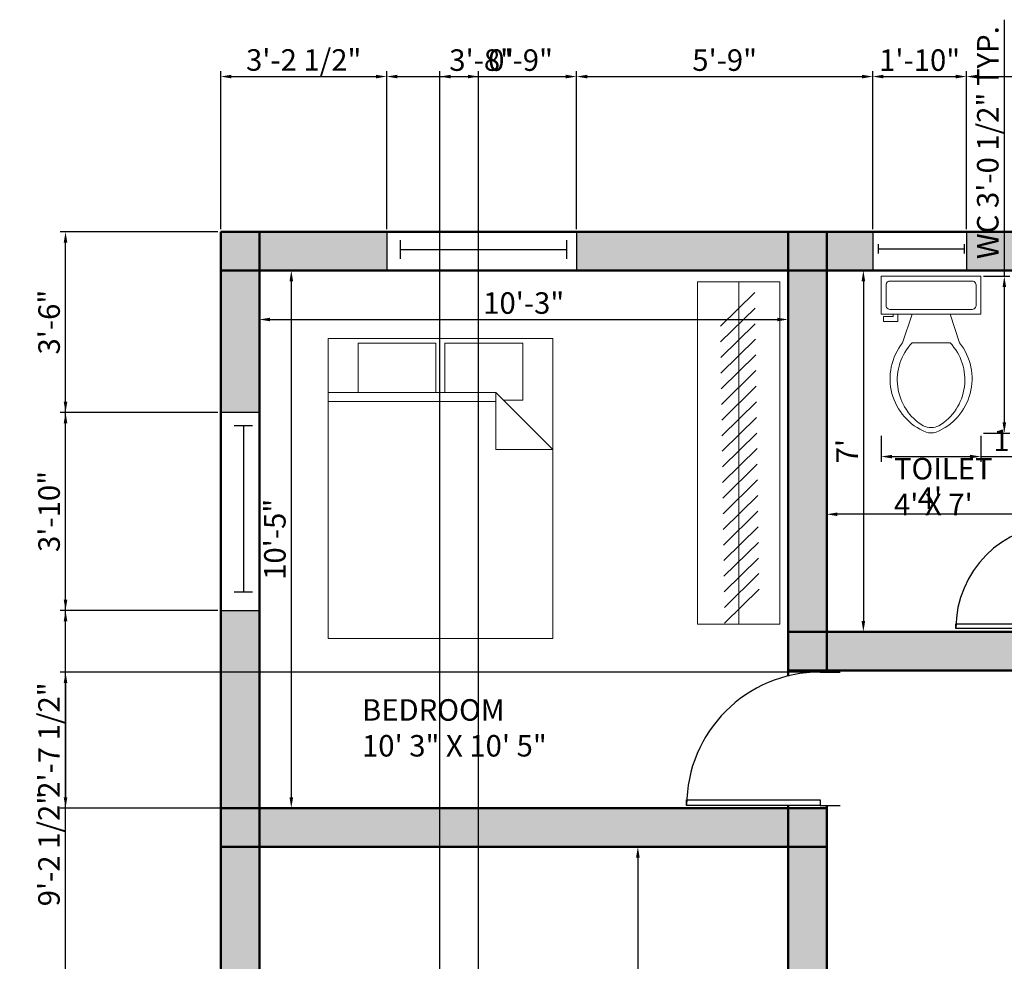
# Model space of a CAD drawing. Units: millimetres. Extents: x 2784 to 3697, y 603 to 1406.
# Tile 3 of 10: x 2784 to 3013, y 1187 to 1406. Entities that reach past the tile are written whole.
import ezdxf

# ---------------------------------------------------------------- set-up
doc = ezdxf.new("R2010")
doc.units = ezdxf.units.MM
for name, color, linetype, lineweight in [('A-ANNO-DIMS', 140, 'Continuous', 18), ('A-AREA-IDEN', 150, 'Continuous', 25), ('A-DOOR', 10, 'Continuous', 25), ('A-FLOR-FIXT', 8, 'Continuous', 18), ('A-FURN', 80, 'Continuous', 18), ('A-GLAZ', 30, 'Continuous', 25), ('A-WALL', 2, 'Continuous', 50), ('A-WALL-PATT', 8, 'Continuous', 13)]:
    doc.layers.add(name, color=color, linetype=linetype, lineweight=lineweight)
doc.styles.get("Standard").update_dxf_attribs({"font": 'arial.ttf'})
doc.dimstyles.new('ISO-25', dxfattribs={"dimtxt": 5, "dimasz": 2.5, "dimexe": 1.25, "dimexo": 0.625, "dimtad": 1, "dimdec": 0, "dimlunit": 3, "dimtxsty": 'Standard', "dimcen": 2.5, "dimadec": 0, "dimazin": 0, "dimtfac": 1, "dimtdec": 0, "dimtmove": 0, "dimatfit": 3, "dimfxl": 1, "dimarcsym": 0})

# ---------------------------------------------------------------- blocks, each defined once
blk = doc.blocks.new('*U2')
for p, q in [((0, 0), (0, -6)), ((40, 0), (40, -6))]:
    blk.add_line(p, q)
blk.add_lwpolyline([(0, 0), (0, 40), (1.75, 40), (1.75, 0)], close=True)
blk.add_arc((0, 0), 40, 0, 90)
blk = doc.blocks.new('*U4')
for p, q in [((0, 4), (0, 0)), ((36, 4), (36, 0)), ((0, 2), (36, 2))]:
    blk.add_line(p, q)
blk = doc.blocks.new('*U5')
for p, q in [((0, 4), (0, 0)), ((0, 2), (36, 2)), ((36, 4), (36, 0))]:
    blk.add_line(p, q)
blk = doc.blocks.new('Bed - Queen')
for p, q in [((0, -80.00003), (0, 0)), ((0, 0), (59.99999, 0)), ((59.99999, 0), (59.99999, -80.00003)), ((7.99999, -1.2), (28.79998, -1.2)), ((7.99999, -14.4), (7.99999, -1.2)), ((28.79998, -1.2), (28.79998, -14.4)), ((31.19999, -1.2), (51.99999, -1.2)), ((31.19999, -14.4), (31.19999, -1.2)), ((51.99999, -1.2), (51.99999, -16.4)), ((0, -14.4), (44.8, -14.4)), ((59.99999, -29.6), (44.8, -14.4)), ((44.8, -14.4), (44.8, -29.6)), ((44.8, -16.8), (0, -16.8)), ((51.99999, -16.4), (46.79936, -16.4)), ((44.8, -29.6), (59.99999, -29.6)), ((59.99999, -80.00003), (0, -80.00003))]:
    blk.add_line(p, q)
blk = doc.blocks.new('Toilet - top')
for p, q in [((9.5, -6), (9.5, -2)), ((-8, -8.5), (-8, -8)), ((-7, -8), (-7, -9.5)), ((-4, -8), (-6, -14)), ((4, -8), (6, -14)), ((-10, -8.5), (-8, -8.5)), ((-10, -9.5), (-10, -8.5)), ((-7, -9.5), (-10, -9.5)), ((4, -14), (-4, -14))]:
    blk.add_line(p, q)
blk.add_lwpolyline([(10.5, -8), (10.5, 0), (-10.5, 0), (-10.5, -8)], close=True)
for points in [[(-9.5, -2), (-9.5, -6)], [(8.5, -1), (-8.5, -1)], [(-8.5, -7), (8.5, -7)]]:
    blk.add_lwpolyline(points)
for centre, radius, start, end in [((-8.62, -1.88), 0.884, 81.8699, 188.1301), ((8.62, -1.88), 0.884, 351.8699, 98.1301), ((-8.62, -6.12), 0.884, 171.8699, 278.1301), ((8.62, -6.12), 0.884, 261.8699, 8.1301), ((3.52, -21.58), 12.17, 141.4691, 247.9714), ((4.2, -21.82), 11.33, 136.3677, 238.9468), ((-3.52, -21.58), 12.17, 292.0284, 38.5307), ((-4.2, -21.82), 11.33, 301.053, 43.6321), ((0, -27.88), 4, 245.7318, 294.2682), ((0, -29), 4, 254.8605, 285.1395)]:
    blk.add_arc(centre, radius, start, end)
blk = doc.blocks.new('*D15')
at = {"layer": 'A-ANNO-DIMS', "color": 0, "lineweight": -2, "transparency": 16777216}
for p, q in [((2847.96, 1347.23), (2848.58, 1347.23)), ((2847.33, 1344.73), (2847.33, 1224.73)), ((2847.96, 1222.23), (2848.58, 1222.23))]:
    blk.add_line(p, q, dxfattribs=at)
at = {"layer": 'A-ANNO-DIMS', "color": 0, "transparency": 16777216}
for points in [[(2846.92, 1344.73), (2847.75, 1344.73), (2847.33, 1347.23)], [(2846.92, 1224.73), (2847.75, 1224.73), (2847.33, 1222.23)]]:
    blk.add_solid(points, dxfattribs=at)
at = {"layer": 'Defpoints', "color": 0, "transparency": 16777216}
for p in [(2847.33, 1347.23), (2847.33, 1222.23), (2847.33, 1222.23)]:
    blk.add_point(p, dxfattribs=at)
at = {"layer": 'A-ANNO-DIMS', "color": 0, "transparency": 16777216, "insert": (2844.16, 1284.73), "char_height": 5, "attachment_point": 5, "rotation": 90}
blk.add_mtext('10\'-5"', dxfattribs=at)
blk = doc.blocks.new('*D16')
at = {"layer": 'A-ANNO-DIMS', "color": 0, "lineweight": -2, "transparency": 16777216}
for p, q in [((2839.91, 1339.59), (2839.91, 1334.59)), ((2962.91, 1339.59), (2962.91, 1334.59)), ((2842.41, 1335.84), (2960.41, 1335.84))]:
    blk.add_line(p, q, dxfattribs=at)
at = {"layer": 'A-ANNO-DIMS', "color": 0, "transparency": 16777216}
for points in [[(2842.41, 1336.26), (2842.41, 1335.43), (2839.91, 1335.84)], [(2960.41, 1336.26), (2960.41, 1335.43), (2962.91, 1335.84)]]:
    blk.add_solid(points, dxfattribs=at)
at = {"layer": 'Defpoints', "color": 0, "transparency": 16777216}
for p in [(2839.91, 1340.22), (2962.91, 1340.22), (2962.91, 1335.84)]:
    blk.add_point(p, dxfattribs=at)
at = {"layer": 'A-ANNO-DIMS', "color": 0, "transparency": 16777216, "insert": (2901.41, 1339.02), "char_height": 5, "attachment_point": 5}
blk.add_mtext('10\'-3"', dxfattribs=at)
blk = doc.blocks.new('*D17')
at = {"layer": 'A-ANNO-DIMS', "color": 0, "lineweight": -2, "transparency": 16777216}
for p, q in [((2975.99, 1347.23), (2981.68, 1347.23)), ((2980.43, 1344.73), (2980.43, 1265.73)), ((2975.99, 1263.23), (2981.68, 1263.23))]:
    blk.add_line(p, q, dxfattribs=at)
at = {"layer": 'A-ANNO-DIMS', "color": 0, "transparency": 16777216}
for points in [[(2980.02, 1344.73), (2980.85, 1344.73), (2980.43, 1347.23)], [(2980.02, 1265.73), (2980.85, 1265.73), (2980.43, 1263.23)]]:
    blk.add_solid(points, dxfattribs=at)
at = {"layer": 'Defpoints', "color": 0, "transparency": 16777216}
for p in [(2975.36, 1347.23), (2975.36, 1263.23), (2980.43, 1263.23)]:
    blk.add_point(p, dxfattribs=at)
at = {"layer": 'A-ANNO-DIMS', "color": 0, "transparency": 16777216, "insert": (2977.31, 1305.23), "char_height": 5, "attachment_point": 5, "rotation": 90}
blk.add_mtext("7'", dxfattribs=at)
blk = doc.blocks.new('*D18')
at = {"layer": 'A-ANNO-DIMS', "color": 0, "lineweight": -2, "transparency": 16777216}
for p, q in [((2971.91, 1291.46), (2971.91, 1289.3)), ((3017.41, 1290.55), (2974.41, 1290.55)), ((3019.91, 1291.46), (3019.91, 1289.3))]:
    blk.add_line(p, q, dxfattribs=at)
at = {"layer": 'A-ANNO-DIMS', "color": 0, "transparency": 16777216}
for points in [[(2974.41, 1290.97), (2974.41, 1290.13), (2971.91, 1290.55)], [(3017.41, 1290.97), (3017.41, 1290.13), (3019.91, 1290.55)]]:
    blk.add_solid(points, dxfattribs=at)
at = {"layer": 'Defpoints', "color": 0, "transparency": 16777216}
for p in [(2971.91, 1292.08), (3019.91, 1292.08), (2971.91, 1290.55)]:
    blk.add_point(p, dxfattribs=at)
at = {"layer": 'A-ANNO-DIMS', "color": 0, "transparency": 16777216, "insert": (2995.91, 1293.67), "char_height": 5, "attachment_point": 5}
blk.add_mtext("4'", dxfattribs=at)
blk = doc.blocks.new('*D21')
at = {"layer": 'A-ANNO-DIMS', "color": 0, "lineweight": -2, "transparency": 16777216}
for p, q in [((2927.49, 1213.23), (2929.22, 1213.23)), ((2927.97, 1210.73), (2927.97, 1044.73)), ((2927.49, 1042.23), (2929.22, 1042.23))]:
    blk.add_line(p, q, dxfattribs=at)
at = {"layer": 'A-ANNO-DIMS', "color": 0, "transparency": 16777216}
for points in [[(2927.55, 1210.73), (2928.39, 1210.73), (2927.97, 1213.23)], [(2927.55, 1044.73), (2928.39, 1044.73), (2927.97, 1042.23)]]:
    blk.add_solid(points, dxfattribs=at)
at = {"layer": 'Defpoints', "color": 0, "transparency": 16777216}
for p in [(2926.87, 1213.23), (2926.87, 1042.23), (2927.97, 1042.23)]:
    blk.add_point(p, dxfattribs=at)
at = {"layer": 'A-ANNO-DIMS', "color": 0, "transparency": 16777216, "insert": (2924.79, 1127.73), "char_height": 5, "attachment_point": 5, "rotation": 90}
blk.add_mtext('14\'-3"', dxfattribs=at)
blk = doc.blocks.new('*D72')
at = {"layer": 'A-ANNO-DIMS', "color": 0, "lineweight": -2, "transparency": 16777216}
for p, q in [((3013.24, 1345.89), (3013.24, 1405.55)), ((3008.39, 1345.89), (3014.49, 1345.89)), ((3013.24, 1311.94), (3013.24, 1343.39)), ((3008.39, 1309.44), (3014.49, 1309.44))]:
    blk.add_line(p, q, dxfattribs=at)
at = {"layer": 'A-ANNO-DIMS', "color": 0, "transparency": 16777216}
for points in [[(3012.82, 1343.39), (3013.65, 1343.39), (3013.24, 1345.89)], [(3012.82, 1311.94), (3013.65, 1311.94), (3013.24, 1309.44)]]:
    blk.add_solid(points, dxfattribs=at)
at = {"layer": 'Defpoints', "color": 0, "transparency": 16777216}
for p in [(3007.77, 1345.89), (3013.24, 1345.89), (3007.77, 1309.44)]:
    blk.add_point(p, dxfattribs=at)
at = {"layer": 'A-ANNO-DIMS', "color": 0, "transparency": 16777216, "insert": (3010.03, 1376.97), "char_height": 5, "attachment_point": 5, "rotation": 90}
blk.add_mtext('WC 3\'-0 1/2" TYP.', dxfattribs=at)
blk = doc.blocks.new('*D73')
at = {"layer": 'A-ANNO-DIMS', "color": 0, "lineweight": -2, "transparency": 16777216}
for p, q in [((2984.6, 1308.81), (2984.6, 1302.72)), ((3007.77, 1308.81), (3007.77, 1302.72)), ((2987.1, 1303.97), (3005.27, 1303.97)), ((3007.77, 1303.97), (3045.41, 1303.97))]:
    blk.add_line(p, q, dxfattribs=at)
at = {"layer": 'A-ANNO-DIMS', "color": 0, "transparency": 16777216}
for points in [[(2987.1, 1304.38), (2987.1, 1303.55), (2984.6, 1303.97)], [(3005.27, 1304.38), (3005.27, 1303.55), (3007.77, 1303.97)]]:
    blk.add_solid(points, dxfattribs=at)
at = {"layer": 'Defpoints', "color": 0, "transparency": 16777216}
for p in [(2984.6, 1309.44), (3007.77, 1309.44), (3007.77, 1303.97)]:
    blk.add_point(p, dxfattribs=at)
at = {"layer": 'A-ANNO-DIMS', "color": 0, "transparency": 16777216, "insert": (3027.84, 1307.1), "char_height": 5, "attachment_point": 5}
blk.add_mtext('1\'-11" TYP.', dxfattribs=at)
blk = doc.blocks.new('*D76')
at = {"layer": 'A-ANNO-DIMS', "color": 0, "lineweight": -2, "transparency": 16777216}
for p, q in [((2830.91, 1356.86), (2830.91, 1393.58)), ((2869.53, 1356.86), (2869.53, 1393.58)), ((2833.41, 1392.33), (2867.03, 1392.33))]:
    blk.add_line(p, q, dxfattribs=at)
at = {"layer": 'A-ANNO-DIMS', "color": 0, "transparency": 16777216}
for points in [[(2833.41, 1392.75), (2833.41, 1391.91), (2830.91, 1392.33)], [(2867.03, 1392.75), (2867.03, 1391.91), (2869.53, 1392.33)]]:
    blk.add_solid(points, dxfattribs=at)
at = {"layer": 'Defpoints', "color": 0, "transparency": 16777216}
for p in [(2869.53, 1392.33), (2830.91, 1356.23), (2869.53, 1356.23)]:
    blk.add_point(p, dxfattribs=at)
at = {"layer": 'A-ANNO-DIMS', "color": 0, "transparency": 16777216, "insert": (2850.22, 1395.54), "char_height": 5, "attachment_point": 5}
blk.add_mtext('3\'-2 1/2"', dxfattribs=at)
blk = doc.blocks.new('*D77')
at = {"layer": 'A-ANNO-DIMS', "color": 0, "lineweight": -2, "transparency": 16777216}
for p, q in [((2869.53, 1356.86), (2869.53, 1393.58)), ((2913.7, 1356.86), (2913.7, 1393.58)), ((2872.03, 1392.33), (2911.2, 1392.33))]:
    blk.add_line(p, q, dxfattribs=at)
at = {"layer": 'A-ANNO-DIMS', "color": 0, "transparency": 16777216}
for points in [[(2872.03, 1392.75), (2872.03, 1391.91), (2869.53, 1392.33)], [(2911.2, 1392.75), (2911.2, 1391.91), (2913.7, 1392.33)]]:
    blk.add_solid(points, dxfattribs=at)
at = {"layer": 'Defpoints', "color": 0, "transparency": 16777216}
for p in [(2913.7, 1392.33), (2869.53, 1356.23), (2913.7, 1356.23)]:
    blk.add_point(p, dxfattribs=at)
at = {"layer": 'A-ANNO-DIMS', "color": 0, "transparency": 16777216, "insert": (2891.62, 1395.51), "char_height": 5, "attachment_point": 5}
blk.add_mtext('3\'-8"', dxfattribs=at)
blk = doc.blocks.new('*D78')
at = {"layer": 'A-ANNO-DIMS', "color": 0, "lineweight": -2, "transparency": 16777216}
for p, q in [((2913.7, 1356.86), (2913.7, 1393.58)), ((2982.62, 1356.86), (2982.62, 1393.58)), ((2916.2, 1392.33), (2980.12, 1392.33))]:
    blk.add_line(p, q, dxfattribs=at)
at = {"layer": 'A-ANNO-DIMS', "color": 0, "transparency": 16777216}
for points in [[(2916.2, 1392.75), (2916.2, 1391.91), (2913.7, 1392.33)], [(2980.12, 1392.75), (2980.12, 1391.91), (2982.62, 1392.33)]]:
    blk.add_solid(points, dxfattribs=at)
at = {"layer": 'Defpoints', "color": 0, "transparency": 16777216}
for p in [(2982.62, 1392.33), (2913.7, 1356.23), (2982.62, 1356.23)]:
    blk.add_point(p, dxfattribs=at)
at = {"layer": 'A-ANNO-DIMS', "color": 0, "transparency": 16777216, "insert": (2948.16, 1395.51), "char_height": 5, "attachment_point": 5}
blk.add_mtext('5\'-9"', dxfattribs=at)
blk = doc.blocks.new('*D79')
at = {"layer": 'A-ANNO-DIMS', "color": 0, "lineweight": -2, "transparency": 16777216}
for p, q in [((2982.62, 1356.86), (2982.62, 1393.58)), ((3004.44, 1356.86), (3004.44, 1393.58)), ((2985.12, 1392.33), (3001.94, 1392.33))]:
    blk.add_line(p, q, dxfattribs=at)
at = {"layer": 'A-ANNO-DIMS', "color": 0, "transparency": 16777216}
for points in [[(2985.12, 1392.75), (2985.12, 1391.91), (2982.62, 1392.33)], [(3001.94, 1392.75), (3001.94, 1391.91), (3004.44, 1392.33)]]:
    blk.add_solid(points, dxfattribs=at)
at = {"layer": 'Defpoints', "color": 0, "transparency": 16777216}
for p in [(3004.44, 1392.33), (2982.62, 1356.23), (3004.44, 1356.23)]:
    blk.add_point(p, dxfattribs=at)
at = {"layer": 'A-ANNO-DIMS', "color": 0, "transparency": 16777216, "insert": (2993.53, 1395.51), "char_height": 5, "attachment_point": 5}
blk.add_mtext('1\'-10"', dxfattribs=at)
blk = doc.blocks.new('*D80')
at = {"layer": 'A-ANNO-DIMS', "color": 0, "lineweight": -2, "transparency": 16777216}
for p, q in [((3004.44, 1356.86), (3004.44, 1393.58)), ((3080.34, 1356.86), (3080.34, 1393.58)), ((3006.94, 1392.33), (3077.84, 1392.33))]:
    blk.add_line(p, q, dxfattribs=at)
at = {"layer": 'A-ANNO-DIMS', "color": 0, "transparency": 16777216}
for points in [[(3006.94, 1392.75), (3006.94, 1391.91), (3004.44, 1392.33)], [(3077.84, 1392.75), (3077.84, 1391.91), (3080.34, 1392.33)]]:
    blk.add_solid(points, dxfattribs=at)
at = {"layer": 'Defpoints', "color": 0, "transparency": 16777216}
for p in [(3080.34, 1392.33), (3004.44, 1356.23), (3080.34, 1356.23)]:
    blk.add_point(p, dxfattribs=at)
at = {"layer": 'A-ANNO-DIMS', "color": 0, "transparency": 16777216, "insert": (3042.39, 1395.51), "char_height": 5, "attachment_point": 5}
blk.add_mtext('6\'-4"', dxfattribs=at)
blk = doc.blocks.new('*D87')
at = {"layer": 'A-ANNO-DIMS', "color": 0, "lineweight": -2, "transparency": 16777216}
for p, q in [((2830.28, 1268.19), (2793.56, 1268.19)), ((2794.81, 1159.96), (2794.81, 1265.69)), ((2830.28, 1157.46), (2793.56, 1157.46))]:
    blk.add_line(p, q, dxfattribs=at)
at = {"layer": 'A-ANNO-DIMS', "color": 0, "transparency": 16777216}
for points in [[(2794.39, 1265.69), (2795.22, 1265.69), (2794.81, 1268.19)], [(2794.39, 1159.96), (2795.22, 1159.96), (2794.81, 1157.46)]]:
    blk.add_solid(points, dxfattribs=at)
at = {"layer": 'Defpoints', "color": 0, "transparency": 16777216}
for p in [(2794.81, 1268.19), (2830.91, 1268.19), (2830.91, 1157.46)]:
    blk.add_point(p, dxfattribs=at)
at = {"layer": 'A-ANNO-DIMS', "color": 0, "transparency": 16777216, "insert": (2791.6, 1212.82), "char_height": 5, "attachment_point": 5, "rotation": 90}
blk.add_mtext('9\'-2 1/2"', dxfattribs=at)
blk = doc.blocks.new('*D88')
at = {"layer": 'A-ANNO-DIMS', "color": 0, "lineweight": -2, "transparency": 16777216}
for p, q in [((2830.28, 1314.23), (2793.56, 1314.23)), ((2794.81, 1270.69), (2794.81, 1311.73)), ((2830.28, 1268.19), (2793.56, 1268.19))]:
    blk.add_line(p, q, dxfattribs=at)
at = {"layer": 'A-ANNO-DIMS', "color": 0, "transparency": 16777216}
for points in [[(2794.39, 1311.73), (2795.22, 1311.73), (2794.81, 1314.23)], [(2794.39, 1270.69), (2795.22, 1270.69), (2794.81, 1268.19)]]:
    blk.add_solid(points, dxfattribs=at)
at = {"layer": 'Defpoints', "color": 0, "transparency": 16777216}
for p in [(2794.81, 1314.23), (2830.91, 1314.23), (2830.91, 1268.19)]:
    blk.add_point(p, dxfattribs=at)
at = {"layer": 'A-ANNO-DIMS', "color": 0, "transparency": 16777216, "insert": (2791.63, 1291.21), "char_height": 5, "attachment_point": 5, "rotation": 90}
blk.add_mtext('3\'-10"', dxfattribs=at)
blk = doc.blocks.new('*D89')
at = {"layer": 'A-ANNO-DIMS', "color": 0, "lineweight": -2, "transparency": 16777216}
for p, q in [((2830.28, 1356.23), (2793.56, 1356.23)), ((2794.81, 1316.73), (2794.81, 1353.73)), ((2830.28, 1314.23), (2793.56, 1314.23))]:
    blk.add_line(p, q, dxfattribs=at)
at = {"layer": 'A-ANNO-DIMS', "color": 0, "transparency": 16777216}
for points in [[(2794.39, 1353.73), (2795.22, 1353.73), (2794.81, 1356.23)], [(2794.39, 1316.73), (2795.22, 1316.73), (2794.81, 1314.23)]]:
    blk.add_solid(points, dxfattribs=at)
at = {"layer": 'Defpoints', "color": 0, "transparency": 16777216}
for p in [(2794.81, 1356.23), (2830.91, 1356.23), (2830.91, 1314.23)]:
    blk.add_point(p, dxfattribs=at)
at = {"layer": 'A-ANNO-DIMS', "color": 0, "transparency": 16777216, "insert": (2791.63, 1335.23), "char_height": 5, "attachment_point": 5, "rotation": 90}
blk.add_mtext('3\'-6"', dxfattribs=at)
blk = doc.blocks.new('*D90')
at = {"layer": 'A-ANNO-DIMS', "color": 0, "lineweight": -2, "transparency": 16777216}
for p, q in [((2830.28, 1356.23), (2793.56, 1356.23)), ((2794.81, 646.1), (2794.81, 1353.73)), ((2830.28, 643.6), (2793.56, 643.6))]:
    blk.add_line(p, q, dxfattribs=at)
at = {"layer": 'A-ANNO-DIMS', "color": 0, "transparency": 16777216}
for points in [[(2794.39, 1353.73), (2795.22, 1353.73), (2794.81, 1356.23)], [(2794.39, 646.1), (2795.22, 646.1), (2794.81, 643.6)]]:
    blk.add_solid(points, dxfattribs=at)
at = {"layer": 'Defpoints', "color": 0, "transparency": 16777216}
for p in [(2794.81, 1356.23), (2830.91, 1356.23), (2830.91, 643.6)]:
    blk.add_point(p, dxfattribs=at)
at = {"layer": 'A-ANNO-DIMS', "color": 0, "transparency": 16777216, "insert": (2791.6, 999.91), "char_height": 5, "attachment_point": 5, "rotation": 90}
blk.add_mtext('59\'-4 1/2"', dxfattribs=at)
blk = doc.blocks.new('*D100')
at = {"layer": 'A-ANNO-DIMS', "color": 0, "lineweight": -2, "transparency": 16777216}
for p, q in [((2971.1, 1253.86), (2793.56, 1253.86)), ((2794.81, 1251.36), (2794.81, 1224.73)), ((2971.28, 1222.23), (2793.56, 1222.23))]:
    blk.add_line(p, q, dxfattribs=at)
at = {"layer": 'A-ANNO-DIMS', "color": 0, "transparency": 16777216}
for points in [[(2794.39, 1251.36), (2795.22, 1251.36), (2794.81, 1253.86)], [(2794.39, 1224.73), (2795.22, 1224.73), (2794.81, 1222.23)]]:
    blk.add_solid(points, dxfattribs=at)
at = {"layer": 'Defpoints', "color": 0, "transparency": 16777216}
for p in [(2971.72, 1253.86), (2794.81, 1222.23), (2971.91, 1222.23)]:
    blk.add_point(p, dxfattribs=at)
at = {"layer": 'A-ANNO-DIMS', "color": 0, "transparency": 16777216, "insert": (2791.6, 1238.05), "char_height": 5, "attachment_point": 5, "rotation": 90}
blk.add_mtext('2\'-7 1/2"', dxfattribs=at)
blk = doc.blocks.new('*D104')
at = {"layer": 'A-ANNO-DIMS', "color": 0, "lineweight": -2, "transparency": 16777216}
for p, q in [((2881.91, 1030.6), (2881.91, 1393.58)), ((2890.91, 1030.6), (2890.91, 1393.58)), ((2884.41, 1392.33), (2888.41, 1392.33)), ((2890.91, 1392.33), (2907.95, 1392.33))]:
    blk.add_line(p, q, dxfattribs=at)
at = {"layer": 'A-ANNO-DIMS', "color": 0, "transparency": 16777216}
for points in [[(2884.41, 1392.75), (2884.41, 1391.91), (2881.91, 1392.33)], [(2888.41, 1392.75), (2888.41, 1391.91), (2890.91, 1392.33)]]:
    blk.add_solid(points, dxfattribs=at)
at = {"layer": 'Defpoints', "color": 0, "transparency": 16777216}
for p in [(2890.91, 1392.33), (2881.91, 1029.97), (2890.91, 1029.97)]:
    blk.add_point(p, dxfattribs=at)
at = {"layer": 'A-ANNO-DIMS', "color": 0, "transparency": 16777216, "insert": (2900.68, 1395.51), "char_height": 5, "attachment_point": 5}
blk.add_mtext('0\'-9"', dxfattribs=at)

msp = doc.modelspace()

# ---------------------------------------------------------------- hatches: boundary and pattern name
at = {"layer": 'A-WALL-PATT'}
h = msp.add_hatch(color=256, dxfattribs=at)
h.dxf.hatch_style = 1
h.paths.add_polyline_path([(2869.53, 1356.23), (2839.91, 1356.23), (2839.91, 1347.23), (2869.53, 1347.23)])
h.paths.add_polyline_path([(2839.91, 1356.23), (2830.91, 1356.23), (2830.91, 1347.23), (2839.91, 1347.23)])
h.paths.add_polyline_path([(2839.91, 1347.23), (2830.91, 1347.23), (2830.91, 1314.23), (2839.91, 1314.23)])
h.paths.add_polyline_path([(2839.91, 1268.19), (2830.91, 1268.19), (2830.91, 1222.23), (2839.91, 1222.23)])
h.paths.add_polyline_path([(2839.91, 1222.23), (2830.91, 1222.23), (2830.91, 1213.23), (2839.91, 1213.23)])
h.paths.add_polyline_path([(2962.91, 1222.23), (2839.91, 1222.23), (2839.91, 1213.23), (2962.91, 1213.23)])
h.paths.add_polyline_path([(2971.91, 1222.23), (2962.91, 1222.23), (2962.91, 1213.23), (2971.91, 1213.23)])
h.paths.add_polyline_path([(2971.91, 1263.23), (2962.91, 1263.23), (2962.91, 1254.23), (2971.91, 1254.23)])
h.paths.add_polyline_path([(2971.91, 1347.23), (2962.91, 1347.23), (2962.91, 1263.23), (2971.91, 1263.23)])
h.paths.add_polyline_path([(2971.91, 1356.23), (2962.91, 1356.23), (2962.91, 1347.23), (2971.91, 1347.23)])
h.paths.add_polyline_path([(2962.91, 1356.23), (2913.7, 1356.23), (2913.7, 1347.23), (2962.91, 1347.23)])
h.paths.add_polyline_path([(2982.62, 1356.23), (2971.91, 1356.23), (2971.91, 1347.23), (2982.62, 1347.23)])
h.paths.add_polyline_path([(3019.91, 1356.23), (3004.44, 1356.23), (3004.44, 1347.23), (3019.91, 1347.23)])
h.paths.add_polyline_path([(3028.91, 1356.23), (3019.91, 1356.23), (3019.91, 1347.23), (3028.91, 1347.23)])
h.paths.add_polyline_path([(3028.91, 1347.23), (3019.91, 1347.23), (3019.91, 1287.35, -0.06506), (3026.12, 1288.16), (3028.91, 1288.16)])
h.paths.add_polyline_path([(3019.91, 1263.23), (2971.91, 1263.23), (2971.91, 1254.23), (3019.91, 1254.23)])
h.paths.add_polyline_path([(3028.91, 1263.23), (3019.91, 1263.23), (3019.91, 1254.23), (3028.91, 1254.23)])
h.paths.add_polyline_path([(3028.91, 1254.23), (3019.91, 1254.23), (3019.91, 1222.23), (3028.91, 1222.23)])
h.paths.add_polyline_path([(3028.91, 1222.23), (3019.91, 1222.23), (3019.91, 1213.23), (3028.91, 1213.23)])
h.paths.add_polyline_path([(3165.91, 1222.23), (3060.65, 1222.23, -0.056956), (3061.45, 1215.23), (3061.45, 1213.23), (3165.91, 1213.23)])
h.paths.add_polyline_path([(3080.34, 1356.23), (3028.91, 1356.23), (3028.91, 1347.23), (3080.34, 1347.23)])
h.paths.add_polyline_path([(3174.91, 1347.23), (3165.91, 1347.23), (3165.91, 1311.28), (3174.91, 1311.28)])
h.paths.add_polyline_path([(3174.91, 1356.23), (3165.91, 1356.23), (3165.91, 1347.23), (3174.91, 1347.23)])
h.paths.add_polyline_path([(3165.91, 1356.23), (3123.1, 1356.23), (3123.1, 1347.23), (3165.91, 1347.23)])
h.paths.add_polyline_path([(3174.91, 1266.65), (3165.91, 1266.65), (3165.91, 1222.23), (3174.91, 1222.23)])
h.paths.add_polyline_path([(3174.91, 1222.23), (3165.91, 1222.23), (3165.91, 1213.23), (3174.91, 1213.23)])
h.paths.add_polyline_path([(3174.91, 1213.23), (3165.91, 1213.23), (3165.91, 1194.83), (3174.91, 1194.83)])
h.paths.add_polyline_path([(3105.91, 1182.92, -0.096276), (3096.91, 1180.92), (3096.91, 1148.23), (3105.91, 1148.23)])
h.paths.add_polyline_path([(3105.91, 1213.23), (3096.91, 1213.23), (3096.91, 1205.07), (3105.91, 1205.07)])
h.paths.add_polyline_path([(2971.91, 1213.23), (2962.91, 1213.23), (2962.91, 1161.09), (2971.91, 1161.09)])
h.paths.add_polyline_path([(2839.91, 1213.23), (2830.91, 1213.23), (2830.91, 1157.46), (2839.91, 1157.46)])
h.paths.add_polyline_path([(2839.91, 1108.88), (2830.91, 1108.88), (2830.91, 1042.23), (2839.91, 1042.23)])
h.paths.add_polyline_path([(2839.91, 1042.23), (2830.91, 1042.23), (2830.91, 1033.23), (2839.91, 1033.23)])
h.paths.add_polyline_path([(2881.91, 1042.23), (2839.91, 1042.23), (2839.91, 1033.23), (2881.91, 1033.23)])
h.paths.add_polyline_path([(2996.91, 1042.23), (2890.91, 1042.23), (2890.91, 1033.23), (2996.91, 1033.23)])
h.paths.add_polyline_path([(2890.91, 1042.23), (2881.91, 1042.23), (2881.91, 1033.23), (2890.91, 1033.23)])
h.paths.add_polyline_path([(2890.91, 1033.23), (2881.91, 1033.23), (2881.91, 984.23), (2890.91, 984.23)])
h.paths.add_polyline_path([(2839.91, 1033.23), (2830.91, 1033.23), (2830.91, 984.23), (2839.91, 984.23)])
h.paths.add_polyline_path([(2839.91, 984.23), (2830.91, 984.23), (2830.91, 975.23), (2839.91, 975.23)])
h.paths.add_polyline_path([(2881.91, 984.23), (2854.14, 984.23, -0.154991), (2857.05, 975.23), (2881.91, 975.23)])
h.paths.add_polyline_path([(2890.91, 984.23), (2881.91, 984.23), (2881.91, 975.23), (2890.91, 975.23)])
h.paths.add_polyline_path([(2900.85, 984.23), (2890.91, 984.23), (2890.91, 975.23), (2900.85, 975.23), (2900.85, 975.78)])
h.paths.add_polyline_path([(2996.91, 984.23), (2923.49, 984.23, -0.089525), (2925.01, 975.78), (2925.01, 975.23), (2996.91, 975.23)])
h.paths.add_polyline_path([(3165.91, 984.23), (3005.91, 984.23), (3005.91, 975.23), (3165.91, 975.23)])
h.paths.add_polyline_path([(3005.91, 1033.23), (2996.91, 1033.23), (2996.91, 984.23), (3005.91, 984.23)])
h.paths.add_polyline_path([(3005.91, 984.23), (2996.91, 984.23), (2996.91, 975.23), (3005.91, 975.23)])
h.paths.add_polyline_path([(3005.91, 1042.23), (2996.91, 1042.23), (2996.91, 1033.23), (3005.91, 1033.23)])
h.paths.add_polyline_path([(3096.91, 1079.23), (2971.91, 1079.23), (2971.91, 1070.23), (3096.91, 1070.23)])
h.paths.add_polyline_path([(2971.91, 1079.23), (2962.91, 1079.23), (2962.91, 1070.23), (2971.91, 1070.23)])
h.paths.add_polyline_path([(2971.91, 1070.23), (2962.91, 1070.23), (2962.91, 1060.28, -0.115005), (2971.91, 1066.55)])
h.paths.add_polyline_path([(2971.91, 1105.54), (2962.91, 1105.54), (2962.91, 1079.23), (2971.91, 1079.23)])
h.paths.add_polyline_path([(3165.91, 1079.23), (3105.91, 1079.23), (3105.91, 1070.23), (3165.91, 1070.23)])
h.paths.add_polyline_path([(3105.91, 1079.23), (3096.91, 1079.23), (3096.91, 1070.23), (3105.91, 1070.23)])
h.paths.add_polyline_path([(3105.91, 1148.23), (3096.91, 1148.23), (3096.91, 1139.23), (3105.91, 1139.23)])
h.paths.add_polyline_path([(3105.91, 1139.23), (3096.91, 1139.23), (3096.91, 1104.7), (3098.08, 1104.75, -0.08216), (3105.91, 1103.81)])
h.paths.add_polyline_path([(3165.91, 1148.23), (3105.91, 1148.23), (3105.91, 1139.23), (3165.91, 1139.23)])
h.paths.add_polyline_path([(3174.91, 1148.23), (3165.91, 1148.23), (3165.91, 1139.23), (3174.91, 1139.23)])
h.paths.add_polyline_path([(3174.91, 1139.23), (3165.91, 1139.23), (3165.91, 1123.86), (3174.91, 1123.86)])
h.paths.add_polyline_path([(3174.91, 1097.37), (3165.91, 1097.37), (3165.91, 1079.23), (3174.91, 1079.23)])
h.paths.add_polyline_path([(3174.91, 1079.23), (3165.91, 1079.23), (3165.91, 1070.23), (3174.91, 1070.23)])
h.paths.add_polyline_path([(3174.91, 1070.23), (3165.91, 1070.23), (3165.91, 1048.77), (3174.91, 1048.77)])
h.paths.add_polyline_path([(3174.91, 1002.74), (3165.91, 1002.74), (3165.91, 984.23), (3174.91, 984.23)])
h.paths.add_polyline_path([(3174.91, 984.23), (3165.91, 984.23), (3165.91, 975.23), (3174.91, 975.23)])
h.paths.add_polyline_path([(3174.91, 975.23), (3165.91, 975.23), (3165.91, 725.23), (3174.91, 725.23)])
h.paths.add_polyline_path([(2839.91, 975.23), (2830.91, 975.23), (2830.91, 725.23), (2839.91, 725.23)])
h.paths.add_polyline_path([(3165.91, 725.23), (2839.91, 725.23), (2839.91, 716.23), (3165.91, 716.23)])
h.paths.add_polyline_path([(3174.91, 725.23), (3165.91, 725.23), (3165.91, 716.23), (3174.91, 716.23)])
h.paths.add_polyline_path([(2839.91, 725.23), (2830.91, 725.23), (2830.91, 716.23), (2839.91, 716.23)])

# ---------------------------------------------------------------- linework, layer by layer
at = {"layer": 'A-FURN'}
for p, q in [((2951.43, 1265.02), (2951.43, 1344.6)), ((2955.17, 1342.13), (2947.16, 1334.26)), ((2955.23, 1338.5), (2947.21, 1330.63)), ((2955.28, 1334.87), (2947.26, 1326.99)), ((2955.33, 1331.24), (2947.31, 1323.36)), ((2955.38, 1327.6), (2947.37, 1319.73)), ((2955.43, 1323.97), (2947.42, 1316.1)), ((2955.49, 1320.34), (2947.47, 1312.46)), ((2955.54, 1316.71), (2947.52, 1308.83)), ((2955.59, 1313.07), (2947.57, 1305.2)), ((2955.64, 1309.44), (2947.63, 1301.57)), ((2955.69, 1305.81), (2947.68, 1297.93)), ((2955.75, 1302.18), (2947.73, 1294.3)), ((2955.8, 1298.54), (2947.78, 1290.67)), ((2955.85, 1294.91), (2947.83, 1287.04)), ((2955.9, 1291.28), (2947.89, 1283.4)), ((2955.95, 1287.65), (2947.94, 1279.77)), ((2956.01, 1284.01), (2947.99, 1276.14)), ((2956.06, 1280.38), (2948.04, 1272.51)), ((2956.11, 1276.75), (2948.09, 1268.87)), ((2956.16, 1273.12), (2948.15, 1265.24))]:
    msp.add_line(p, q, dxfattribs=at)
msp.add_lwpolyline([(2961.01, 1344.6), (2941.85, 1344.6), (2941.85, 1265.02), (2961.01, 1265.02)], close=True, dxfattribs=at)
at = {"layer": 'A-GLAZ'}
for p, q in [((2869.53, 1356.23), (2869.53, 1347.23)), ((2913.7, 1356.23), (2913.7, 1347.23)), ((2982.62, 1356.23), (2982.62, 1347.23)), ((3004.44, 1356.23), (3004.44, 1347.23)), ((2839.91, 1314.23), (2830.91, 1314.23)), ((2830.91, 1268.19), (2839.91, 1268.19))]:
    msp.add_line(p, q, dxfattribs=at)
at = {"layer": 'A-WALL'}
for p, q in [((2830.91, 1356.23), (2830.91, 716.23)), ((2830.91, 1356.23), (3174.91, 1356.23)), ((2839.91, 1356.23), (2839.91, 643.6)), ((2962.91, 1356.23), (2962.91, 1252.95)), ((2962.91, 1356.23), (2962.91, 1252.95)), ((2971.91, 1356.23), (2971.91, 1253.86)), ((2971.91, 1356.23), (2971.91, 1253.86)), ((2830.91, 1347.23), (3174.91, 1347.23)), ((2962.91, 1263.23), (3028.91, 1263.23)), ((2962.91, 1254.23), (3028.91, 1254.23)), ((2830.91, 1222.23), (2971.91, 1222.23)), ((2830.91, 1222.23), (2971.91, 1222.23)), ((2962.91, 1222.82), (2962.91, 1213.23)), ((2962.91, 1222.82), (2962.91, 1161.09)), ((2971.91, 1222.82), (2971.91, 1213.23)), ((2971.91, 1222.82), (2971.91, 1161.09)), ((2830.91, 1213.23), (2971.91, 1213.23)), ((2830.91, 1213.23), (2971.91, 1213.23))]:
    msp.add_line(p, q, dxfattribs=at)

# ---------------------------------------------------------------- block references
at = {"layer": 'A-DOOR', "rotation": 90}
for p, xscale, yscale, zscale in [((3026.12, 1263.99), 0.6041131756153701, 0.6041131756153701, 0.6041131756153701), ((2970.36, 1222.82), 0.7759495368129277, 0.7759495368129277, 0.7759495368129277)]:
    msp.add_blockref('*U2', p, dxfattribs=dict(at, xscale=xscale, yscale=yscale, zscale=zscale))
at = {"layer": 'A-FLOR-FIXT', "xscale": 1.103188224763309, "yscale": 1.103188224763309, "zscale": 1.103188224763309}
msp.add_blockref('Toilet - top', (2996.19, 1345.89), dxfattribs=at)
at = {"layer": 'A-FURN', "xscale": 0.8718255544036225, "yscale": 0.8718255544036225, "zscale": 0.8718255544036225}
msp.add_blockref('Bed - Queen', (2855.89, 1331.42), dxfattribs=at)
at = {"layer": 'A-GLAZ'}
for name, p, xscale, yscale, zscale in [('*U4', (2872.69, 1349.98), 1.074021802203067, 1.074021802203067, 1.074021802203067), ('*U5', (2983.9, 1351.16), 0.5552882983770857, 0.5552882983770857, 0.5552882983770857)]:
    msp.add_blockref(name, p, dxfattribs=dict(at, xscale=xscale, yscale=yscale, zscale=zscale))
at = {"layer": 'A-GLAZ', "xscale": 1.074021802203067, "yscale": 1.074021802203067, "zscale": 1.074021802203067, "rotation": 270}
msp.add_blockref('*U4', (2834.03, 1311.12), dxfattribs=at)

# ---------------------------------------------------------------- texts
at = {"layer": 'A-AREA-IDEN', "char_height": 5, "attachment_point": 1}
for s, width, insert in [("TOILET \\P4' X 7'", 18.8777, (2987.55, 1303.66)), ('BEDROOM \\P10\' 3" X 10\' 5"', 52.7124, (2863.78, 1247.56))]:
    msp.add_mtext_dynamic_manual_height_columns(s, width=width, gutter_width=12.5, heights=[0], dxfattribs=dict(at, insert=insert))

# ---------------------------------------------------------------- dimensions: what is measured, and where the dimension line sits
at = {"layer": 'A-ANNO-DIMS'}
dim = msp.add_linear_dim(base=(3013.2382, 1345.8915), p1=(3007.7698, 1309.4352), p2=(3007.7698, 1345.8915), angle=90, text='WC <> TYP.', dimstyle='ISO-25', override={"dimdec": 1, "dimrnd": 0, "dimzin": 1, "dimlunit": 4, "dimfrac": 2}, dxfattribs=at)
dim.commit()
dim.dimension.update_dxf_attribs({"geometry": '*D72', "text_midpoint": (3010.0262, 1376.9718)})
for base, p1, p2, override, picture, middle in [((2869.53, 1392.33), (2830.91, 1356.23), (2869.53, 1356.23), {"dimdec": 1, "dimlfac": 1, "dimrnd": 0, "dimzin": 1, "dimdsep": 46, "dimlunit": 4, "dimfrac": 2}, '*D76', (2850.22, 1395.54)), ((2913.7, 1392.33), (2869.53, 1356.23), (2913.7, 1356.23), {"dimdec": 1, "dimlfac": 1, "dimrnd": 0, "dimzin": 1, "dimdsep": 46, "dimlunit": 4, "dimfrac": 2}, '*D77', (2891.62, 1395.51)), ((2890.91, 1392.33), (2881.91, 1029.97), (2890.91, 1029.97), {"dimdec": 1, "dimlfac": 1, "dimrnd": 0, "dimzin": 1, "dimdsep": 46, "dimlunit": 4, "dimfrac": 2}, '*D104', (2900.68, 1395.51)), ((2982.62, 1392.33), (2913.7, 1356.23), (2982.62, 1356.23), {"dimdec": 1, "dimlfac": 1, "dimrnd": 0, "dimzin": 1, "dimdsep": 46, "dimlunit": 4, "dimfrac": 2}, '*D78', (2948.16, 1395.51)), ((3004.44, 1392.33), (2982.62, 1356.23), (3004.44, 1356.23), {"dimdec": 1, "dimlfac": 1, "dimrnd": 0, "dimzin": 1, "dimdsep": 46, "dimlunit": 4, "dimfrac": 2}, '*D79', (2993.53, 1395.51)), ((3080.34, 1392.33), (3004.44, 1356.23), (3080.34, 1356.23), {"dimdec": 1, "dimlfac": 1, "dimrnd": 0, "dimzin": 1, "dimdsep": 46, "dimlunit": 4, "dimfrac": 2}, '*D80', (3042.39, 1395.51)), ((2962.91, 1335.84), (2839.91, 1340.22), (2962.91, 1340.22), {"dimclrd": 0, "dimclre": 0, "dimclrt": 0}, '*D16', (2901.41, 1339.02)), ((2971.91, 1290.55), (3019.91, 1292.08), (2971.91, 1292.08), {"dimclrd": 0, "dimclre": 0, "dimclrt": 0}, '*D18', (2995.91, 1293.67))]:
    dim = msp.add_linear_dim(base=base, p1=p1, p2=p2, dimstyle='ISO-25', override=override, dxfattribs=at)
    dim.commit()
    dim.dimension.update_dxf_attribs({"geometry": picture, "text_midpoint": middle})
for base, p1, p2, override, picture, middle in [((2794.81, 1356.23), (2830.91, 643.6), (2830.91, 1356.23), {"dimdec": 1, "dimlfac": 1, "dimrnd": 0, "dimzin": 1, "dimdsep": 46, "dimlunit": 4, "dimfrac": 2}, '*D90', (2791.6, 999.91)), ((2794.81, 1356.23), (2830.91, 1314.23), (2830.91, 1356.23), {"dimdec": 1, "dimlfac": 1, "dimrnd": 0, "dimzin": 1, "dimdsep": 46, "dimlunit": 4, "dimfrac": 2}, '*D89', (2791.63, 1335.23)), ((2847.33, 1222.23), (2847.33, 1347.23), (2847.33, 1222.23), {"dimclrd": 0, "dimclre": 0, "dimclrt": 0}, '*D15', (2844.16, 1284.73)), ((2980.43, 1263.23), (2975.36, 1347.23), (2975.36, 1263.23), {"dimclrd": 0, "dimclre": 0, "dimclrt": 0}, '*D17', (2977.31, 1305.23)), ((2794.81, 1314.23), (2830.91, 1268.19), (2830.91, 1314.23), {"dimdec": 1, "dimlfac": 1, "dimrnd": 0, "dimzin": 1, "dimdsep": 46, "dimlunit": 4, "dimfrac": 2}, '*D88', (2791.63, 1291.21)), ((2794.81, 1268.19), (2830.91, 1157.46), (2830.91, 1268.19), {"dimdec": 1, "dimlfac": 1, "dimrnd": 0, "dimzin": 1, "dimdsep": 46, "dimlunit": 4, "dimfrac": 2}, '*D87', (2791.6, 1212.82)), ((2794.81, 1222.23), (2971.72, 1253.86), (2971.91, 1222.23), {"dimdec": 1, "dimlfac": 1, "dimrnd": 0, "dimzin": 1, "dimdsep": 46, "dimlunit": 4, "dimfrac": 2}, '*D100', (2791.6, 1238.05)), ((2927.97, 1042.23), (2926.87, 1213.23), (2926.87, 1042.23), {"dimclrd": 0, "dimclre": 0, "dimclrt": 0}, '*D21', (2924.79, 1127.73))]:
    dim = msp.add_linear_dim(base=base, p1=p1, p2=p2, angle=90, dimstyle='ISO-25', override=override, dxfattribs=at)
    dim.commit()
    dim.dimension.update_dxf_attribs({"geometry": picture, "text_midpoint": middle})
dim = msp.add_linear_dim(base=(3007.77, 1303.97), p1=(2984.6, 1309.44), p2=(3007.77, 1309.44), text='<> TYP.', dimstyle='ISO-25', override={"dimdec": 1, "dimrnd": 0, "dimzin": 1, "dimlunit": 4, "dimfrac": 2}, dxfattribs=at)
dim.commit()
dim.dimension.update_dxf_attribs({"geometry": '*D73', "text_midpoint": (3027.84, 1307.1)})

doc.saveas('drawing.dxf')
